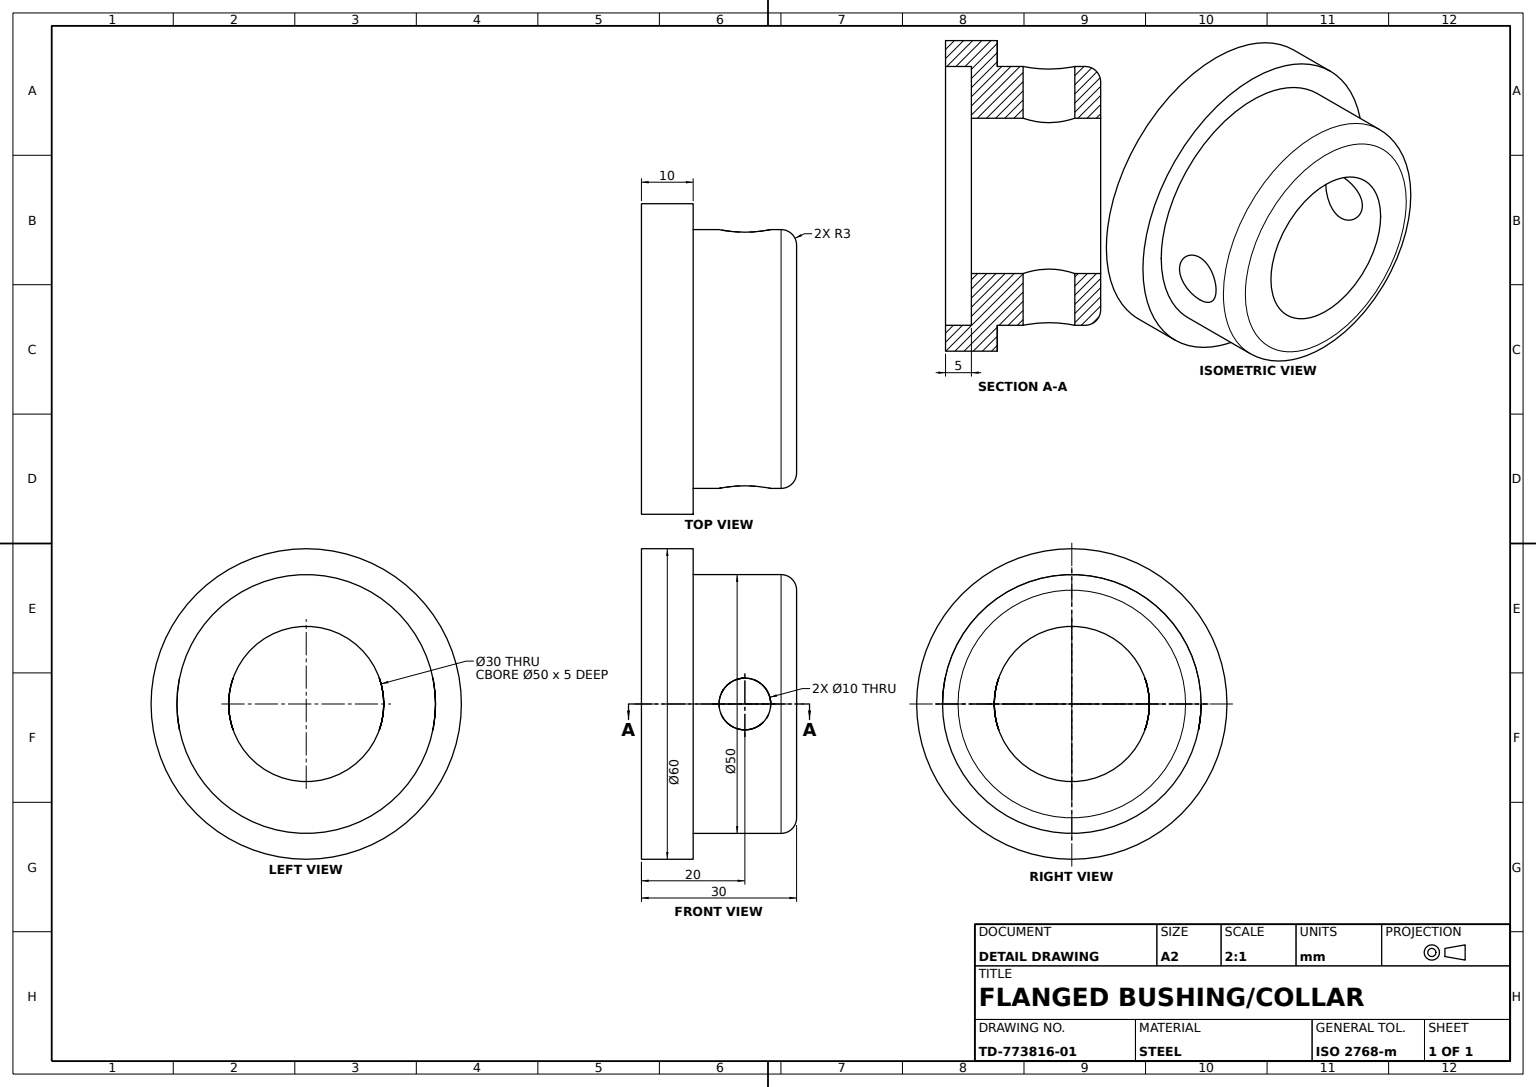
SolidWorks part; units mm, degrees
material "Plain Carbon Steel"
ref_plane "Front Plane" through (0, 0, 0) normal (0, 0, 1) x (1, 0, 0)
ref_plane "Top Plane" through (0, 0, 0) normal (0, 1, 0) x (1, 0, 0)
ref_plane "Right Plane" through (0, 0, 0) normal (1, 0, 0) x (0, 0, -1)
sketch "Flange Profile Ø60" plane through (0, 0, 0) normal (0, 1, 0) x (1, 0, 0)
  circle A0 centre (0, 0) radius 30
  dimension "D1" = 60
extrude "Base Flange Ø60x10" add sketch "Flange Profile Ø60" along normal blind 10
sketch "Boss Profile Ø50" plane through (0, 10, 0) normal (0, 1, 0) x (1, 0, 0)
  circle A0 centre (0, 0) radius 25
  dimension "D1" = 50
extrude "Collar Boss Ø50x20" add sketch "Boss Profile Ø50" along normal blind 20
fillet "Boss Edge Fillet R3" radius 3 1 edges at (0, 30, 25)
sketch "Cross Hole Profile Ø10" plane through (0, 0, 0) normal (0, 0, 1) x (1, 0, 0)
  line L0 (-30, 0) -> (30, 0) construction
  circle A0 centre (0, 20) radius 5
  dimension "D1" = 10
  dimension "D2" = 20
extrude "Cross Hole Ø10" cut sketch "Cross Hole Profile Ø10" against normal mid plane 70
sketch "Counterbore Profile Ø50" plane through (0, 0, 0) normal (0, -1, 0) x (1, 0, 0)
  circle A0 centre (0, 0) radius 25
  dimension "D1" = 50
extrude "Counterbore Ø50x5" cut sketch "Counterbore Profile Ø50" against normal blind 5
sketch "Bore Profile Ø30" plane through (0, 5, 0) normal (0, -1, 0) x (1, 0, 0)
  circle A0 centre (0, 0) radius 15
  dimension "D1" = 30
extrude "Through Bore Ø30" cut sketch "Bore Profile Ø30" against normal blind 94
